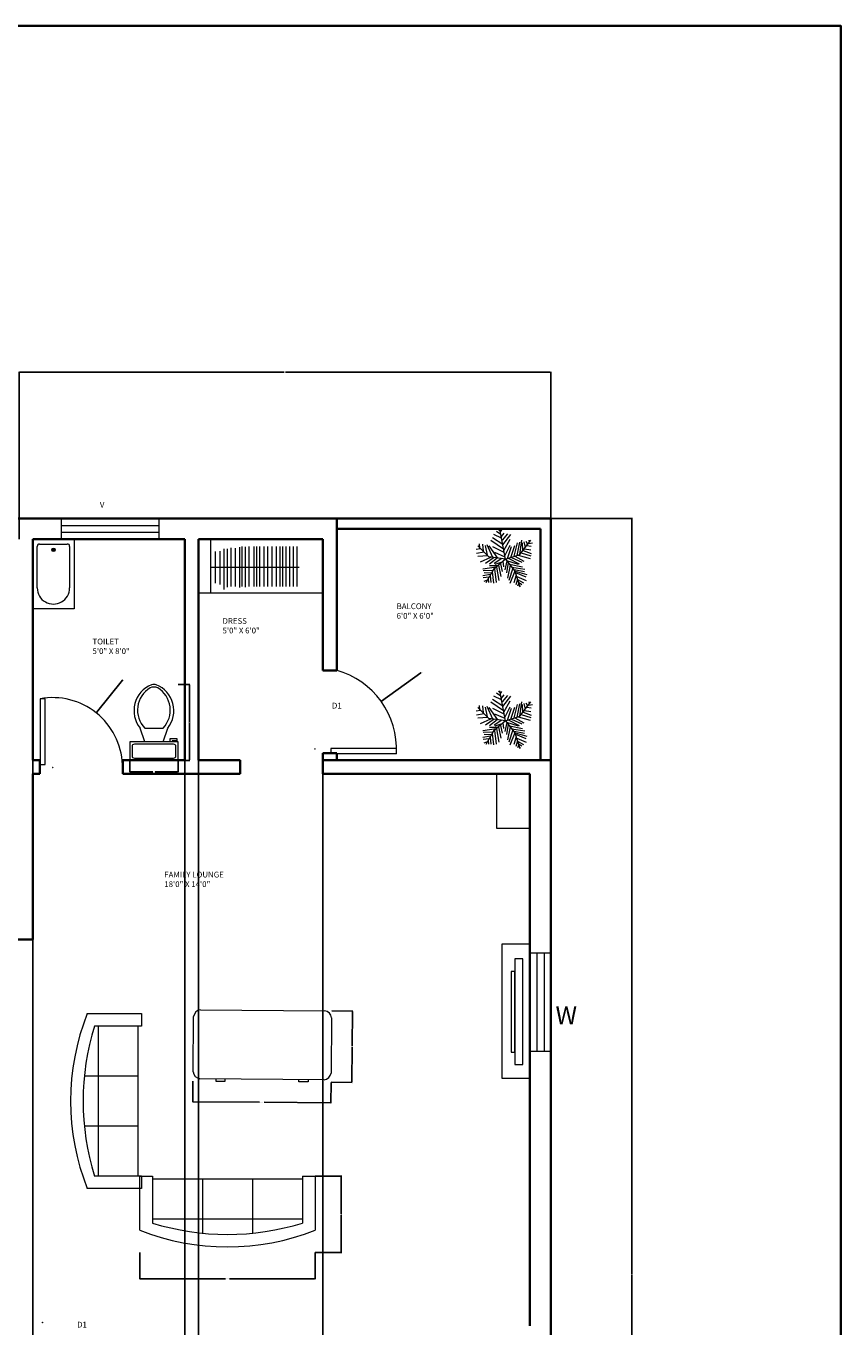
# Model space of a CAD drawing. Units: inches. Extents: x 65 to 1274, y 42 to 1041.
# Tile 6 of 6: x 920 to 1274, y 476 to 1041. Entities that reach past the tile are written whole.
import ezdxf

# ---------------------------------------------------------------- set-up
doc = ezdxf.new("R2010")
doc.units = ezdxf.units.IN
for name, color, linetype, lineweight in [('A-ANNO-DIMS', 2, 'Continuous', 18), ('A-AREA-IDEN', 7, 'Continuous', 18), ('A-DOOR', 3, 'Continuous', 18), ('A-FLOR-CASE', 8, 'Continuous', 18), ('A-FLOR-FIXT', 9, 'Continuous', 18), ('A-FURN', 8, 'Continuous', 18), ('A-GLAZ', 4, 'Continuous', 18), ('A-WALL', 7, 'Continuous', 35), ('L-PLNT', 94, 'Continuous', 13), ('Text', 7, 'Continuous', 18), ('Title Block', 7, 'Continuous', 35)]:
    doc.layers.add(name, color=color, linetype=linetype, lineweight=lineweight)
doc.styles.get("Standard").update_dxf_attribs({"font": 'arial.ttf'})
doc.dimstyles.get("Standard").update_dxf_attribs({"dimtxt": 0.18, "dimasz": 0.18, "dimexe": 0.18, "dimexo": 0.0625, "dimgap": 0.09, "dimtad": 0, "dimtih": 1, "dimtoh": 1, "dimdec": 4, "dimzin": 0, "dimdsep": 46, "dimtxsty": 'Standard', "dimcen": 0.09, "dimadec": 0, "dimazin": 0, "dimtfac": 1, "dimtdec": 4, "dimtofl": 0, "dimtmove": 0, "dimatfit": 3, "dimfxl": 1, "dimtolj": 1, "dimtzin": 0, "dimarcsym": 0})

# ---------------------------------------------------------------- blocks, each defined once
blk = doc.blocks.new('Toilet - top')
for p, q in [((9.5, -6), (9.5, -2)), ((-10, -8.5), (-8, -8.5)), ((-10, -9.5), (-10, -8.5)), ((-7, -9.5), (-10, -9.5)), ((-8, -8.5), (-8, -8)), ((-7, -8), (-7, -9.5)), ((-4, -8), (-6, -14)), ((4, -8), (6, -14)), ((4, -14), (-4, -14))]:
    blk.add_line(p, q)
blk.add_lwpolyline([(10.5, -8), (10.5, 0), (-10.5, 0), (-10.5, -8)], close=True)
for points in [[(-9.5, -2), (-9.5, -6)], [(8.5, -1), (-8.5, -1)], [(-8.5, -7), (8.5, -7)]]:
    blk.add_lwpolyline(points)
for centre, radius, start, end in [((-8.62, -1.88), 0.884, 81.8699, 188.1301), ((8.62, -1.88), 0.884, 351.8699, 98.1301), ((-8.62, -6.12), 0.884, 171.8699, 278.1301), ((8.62, -6.12), 0.884, 261.8699, 8.1301), ((3.52, -21.58), 12.17, 141.4691, 247.9714), ((4.2, -21.82), 11.33, 136.3677, 238.9468), ((-3.52, -21.58), 12.17, 292.0284, 38.5307), ((-4.2, -21.82), 11.33, 301.053, 43.6321), ((0, -27.88), 4, 245.7318, 294.2682), ((0, -29), 4, 254.8605, 285.1395)]:
    blk.add_arc(centre, radius, start, end)
blk = doc.blocks.new('Bath Tub - 26 x 60 in.')
for p, q in [((8, -18), (10, -18)), ((9, -17), (9, -19))]:
    blk.add_line(p, q)
blk.add_lwpolyline([(0, -36), (0, 0), (60, 0), (60, -36)], close=True)
for points in [[(4, -30), (4, -6)], [(6, -4), (42, -4)], [(42, -32), (6, -32)]]:
    blk.add_lwpolyline(points)
for radius in [1.5, 1]:
    blk.add_circle((9, -18), radius)
for centre, radius, start, end in [((5.75, -5.75), 1.77, 81.8699, 188.1301), ((42, -18), 14, 270, 90), ((5.75, -30.25), 1.77, 171.8699, 278.1301)]:
    blk.add_arc(centre, radius, start, end)
blk = doc.blocks.new('Sofa - Roundback 7 ft.')
for p, q in [((-36.000027, -34), (-36.000027, -11.4696)), ((-12.00002, -32.4421), (-12.00003, -6.5971)), ((11.99997, -32.4421), (11.99998, -6.5971)), ((35.99998, -34), (35.99998, -11.4696)), ((-35.999844, -13.3819), (35.9998, -13.3819)), ((-36.000027, -32.4421), (35.99998, -32.4421))]:
    blk.add_line(p, q)
for points in [[(-36.000027, -34), (-42.000027, -34), (-42.000027, -8)], [(41.99998, -8), (41.99998, -34), (35.99998, -34)]]:
    blk.add_lwpolyline(points)
for centre, radius, start, end in [((0, -114.25), 114.25, 68.43141, 111.5686), ((-0.00001, -127.1968), 121.1968, 72.72033, 107.2797)]:
    blk.add_arc(centre, radius, start, end)
blk = doc.blocks.new('Desk - 30 x 60 in.')
for p, q in [((-26.999995, 0), (26.999995, 0)), ((-29.999995, -27), (-29.999995, -3)), ((29.999995, -3), (29.999995, -27)), ((26.999995, -30), (-26.999995, -30)), ((-20.000005, -30), (-20.000005, -31)), ((-20.000005, -31), (-16.000005, -31)), ((-16.000005, -31), (-16.000005, -30)), ((15.999995, -31), (15.999995, -30)), ((19.999995, -31), (15.999995, -31)), ((19.999995, -30), (19.999995, -31))]:
    blk.add_line(p, q)
for centre, start, end in [((-26.499995, -3.5), 98.1301, 171.8699), ((26.499995, -3.5), 8.130102, 81.8699), ((-26.499995, -26.5), 188.1301, 261.8699), ((26.499995, -26.5), 278.1301, 351.8699)]:
    blk.add_arc(centre, 3.535534, start, end)
blk = doc.blocks.new('*U4')
for p, q in [((-8.737, 47.138), (-17.069, 52.711)), ((-10.186, 53.64), (-13.084, 55.962)), ((0, 0), (-10.5, 57)), ((-9.099, 51.782), (-6.563, 55.962)), ((-7.65, 43.423), (-2.578, 49.46)), ((-31.5, 4.5), (-52.5, 25.5)), ((-48.585, 21.131), (-49.309, 29.026)), ((-43.513, 28.561), (-42.427, 15.558)), ((-38.442, 26.239), (-34.819, 7.663)), ((-35.544, 28.097), (-24.314, 3.947)), ((-14.533, 2.09), (-30.834, 25.31)), ((-3.665, 19.273), (-27.574, 35.527)), ((-5.114, 28.097), (-24.676, 40.636)), ((-7.288, 39.707), (-21.778, 46.673)), ((-5.839, 35.992), (4.667, 48.067)), ((-5.114, 27.632), (10.463, 46.673)), ((-2.941, 16.486), (8.652, 37.85)), ((-1.129, 6.734), (9.014, 26.704)), ((10.101, 3.483), (17.708, 26.239)), ((16.259, 5.805), (23.142, 31.348)), ((22.055, 7.198), (27.489, 32.277)), ((27, 9), (48, 36)), ((27.127, 9.056), (31.112, 35.992)), ((31.836, 30.883), (32.561, 16.486)), ((35.096, 32.741), (37.27, 22.524)), ((38.719, 34.134), (41.979, 28.561)), ((40.53, 25.775), (48.862, 24.846)), ((43.791, 29.954), (51.036, 30.883)), ((44.153, 36.456), (45.239, 32.741)), ((-47.498, 19.737), (-55.83, 18.344)), ((-40.615, 13.7), (-55.105, 10.913)), ((-33.37, 6.269), (-52.207, 5.34)), ((-28.299, 3.483), (-47.86, -5.805)), ((-21.416, 3.018), (-38.079, -8.128)), ((0, 0), (-31.5, 4.5)), ((-15.982, 2.09), (-30.11, -9.521)), ((-24.314, 23.917), (-2.941, 13.7)), ((0, 0), (-22.5, -19.5)), ((-6.563, 1.161), (-21.416, -8.128)), ((-20.691, 13.7), (-1.129, 4.876)), ((0, 0), (27, 9)), ((0, 0), (18, -22.5)), ((3.942, 1.625), (11.187, 24.381)), ((6.478, 1.625), (26.04, -8.592)), ((11.187, 3.483), (30.749, -5.805)), ((18.07, 5.805), (35.096, -3.483)), ((24.229, 7.663), (46.688, 1.625)), ((29.662, 12.307), (48.137, 6.269)), ((33.285, 16.486), (48.862, 10.913)), ((36.183, 19.737), (48.137, 17.88)), ((-17.431, -15.094), (-42.789, -18.809)), ((-24.314, -21.596), (-42.427, -22.06)), ((-22.5, -19.5), (-37.5, -45)), ((-15.257, -12.772), (-30.11, -12.772)), ((-25.038, -23.918), (-22.865, -45.281)), ((-20.691, -18.345), (-17.793, -44.352)), ((-6.563, -5.805), (-19.967, -9.985)), ((-17.069, -15.094), (-12.721, -40.172)), ((-13.446, -11.378), (-8.737, -32.741)), ((-9.461, -8.592), (-6.201, -23.453)), ((-4.752, -3.483), (-3.665, -14.629)), ((2.493, -3.019), (-1.491, -20.202)), ((1.769, -2.555), (24.229, -9.521)), ((5.029, -6.27), (2.131, -25.775)), ((9.014, -11.378), (3.58, -35.992)), ((14.085, -16.951), (6.478, -40.172)), ((7.565, -9.056), (32.198, -14.629)), ((18.07, -22.524), (8.289, -45.745)), ((12.274, -15.094), (36.907, -18.809)), ((16.259, -19.738), (36.183, -22.989)), ((18, -22.5), (27, -52.5)), ((18.433, -22.524), (40.53, -29.026)), ((-28.299, -29.026), (-42.789, -31.348)), ((-30.834, -34.135), (-42.427, -35.528)), ((-34.457, -39.708), (-40.978, -42.494)), ((-26.849, -26.24), (-40.253, -25.775)), ((-32.646, -36.921), (-31.921, -44.352)), ((-29.023, -30.884), (-27.936, -43.887)), ((20.244, -30.419), (15.897, -44.816)), ((19.157, -25.311), (38.719, -33.206)), ((22.78, -37.85), (19.519, -48.532)), ((21.331, -32.741), (39.081, -40.636)), ((22.78, -38.314), (34.372, -44.816)), ((24.591, -45.745), (23.142, -50.854)), ((24.591, -43.423), (30.749, -47.603)), ((26.764, -49.925), (28.213, -50.854))]:
    blk.add_line(p, q)
blk = doc.blocks.new('WIN-43-DEEP-FRAME')
for p, q in [((9, 42.65), (0, 42.65)), ((0, 42.65), (0, 0)), ((3, 0), (3, 42.65)), ((6, 42.65), (6, 0)), ((9, 0), (9, 42.65)), ((0, 0), (9, 0))]:
    blk.add_line(p, q)
blk = doc.blocks.new('*D36')
at = {"layer": 'A-ANNO-DIMS', "color": 0, "lineweight": -2, "transparency": 16777216}
for p, q in [((969.32, 508.05), (969.32, 496.52)), ((1045.42, 508.05), (1045.42, 496.52)), ((969.5, 496.7), (1006.47, 496.7)), ((1045.24, 496.7), (1008.28, 496.7))]:
    blk.add_line(p, q, dxfattribs=at)
at = {"layer": 'A-ANNO-DIMS', "color": 0, "transparency": 16777216}
for points in [[(969.5, 496.73), (969.5, 496.67), (969.32, 496.7)], [(1045.24, 496.73), (1045.24, 496.67), (1045.42, 496.7)]]:
    blk.add_solid(points, dxfattribs=at)
at = {"layer": 'Defpoints', "color": 0, "transparency": 16777216}
for p in [(969.32, 508.11), (1045.42, 508.11), (969.32, 496.7)]:
    blk.add_point(p, dxfattribs=at)
at = {"layer": 'A-ANNO-DIMS', "color": 0, "transparency": 16777216, "insert": (1007.37, 496.7), "char_height": 0.18, "attachment_point": 5}
blk.add_mtext('\\A1;SOFA 76 TYP.', dxfattribs=at)
blk = doc.blocks.new('*D37')
at = {"layer": 'A-ANNO-DIMS', "color": 0, "lineweight": -2, "transparency": 16777216}
for p, q in [((1045.48, 541.33), (1057.02, 541.33)), ((1056.84, 541.15), (1056.84, 524.91)), ((1056.84, 508.29), (1056.84, 524.54)), ((1045.48, 508.11), (1057.02, 508.11))]:
    blk.add_line(p, q, dxfattribs=at)
at = {"layer": 'A-ANNO-DIMS', "color": 0, "transparency": 16777216}
for points in [[(1056.81, 541.15), (1056.87, 541.15), (1056.84, 541.33)], [(1056.81, 508.29), (1056.87, 508.29), (1056.84, 508.11)]]:
    blk.add_solid(points, dxfattribs=at)
at = {"layer": 'Defpoints', "color": 0, "transparency": 16777216}
for p in [(1045.42, 541.33), (1045.42, 508.11), (1056.84, 508.11)]:
    blk.add_point(p, dxfattribs=at)
at = {"layer": 'A-ANNO-DIMS', "color": 0, "transparency": 16777216, "insert": (1056.84, 524.72), "char_height": 0.18, "attachment_point": 5}
blk.add_mtext('\\A1;33 TYP.', dxfattribs=at)
blk = doc.blocks.new('*D40')
at = {"layer": 'A-ANNO-DIMS', "color": 0, "lineweight": -2, "transparency": 16777216}
for p, q in [((985.96, 755.09), (991.04, 755.09)), ((990.86, 754.91), (990.86, 738.75)), ((990.86, 722.22), (990.86, 738.38)), ((985.96, 722.04), (991.04, 722.04))]:
    blk.add_line(p, q, dxfattribs=at)
at = {"layer": 'A-ANNO-DIMS', "color": 0, "transparency": 16777216}
for points in [[(990.83, 754.91), (990.89, 754.91), (990.86, 755.09)], [(990.83, 722.22), (990.89, 722.22), (990.86, 722.04)]]:
    blk.add_solid(points, dxfattribs=at)
at = {"layer": 'Defpoints', "color": 0, "transparency": 16777216}
for p in [(985.9, 755.09), (985.9, 722.04), (990.86, 722.04)]:
    blk.add_point(p, dxfattribs=at)
at = {"layer": 'A-ANNO-DIMS', "color": 0, "transparency": 16777216, "insert": (990.86, 738.56), "char_height": 0.18, "attachment_point": 5}
blk.add_mtext('\\A1;WC 33 TYP.', dxfattribs=at)
blk = doc.blocks.new('*D41')
at = {"layer": 'A-ANNO-DIMS', "color": 0, "lineweight": -2, "transparency": 16777216}
for p, q in [((964.9, 721.98), (964.9, 716.9)), ((985.9, 721.98), (985.9, 716.9)), ((965.08, 717.08), (974.87, 717.08)), ((985.72, 717.08), (975.93, 717.08))]:
    blk.add_line(p, q, dxfattribs=at)
at = {"layer": 'A-ANNO-DIMS', "color": 0, "transparency": 16777216}
for points in [[(965.08, 717.11), (965.08, 717.05), (964.9, 717.08)], [(985.72, 717.11), (985.72, 717.05), (985.9, 717.08)]]:
    blk.add_solid(points, dxfattribs=at)
at = {"layer": 'Defpoints', "color": 0, "transparency": 16777216}
for p in [(964.9, 722.04), (985.9, 722.04), (964.9, 717.08)]:
    blk.add_point(p, dxfattribs=at)
at = {"layer": 'A-ANNO-DIMS', "color": 0, "transparency": 16777216, "insert": (975.4, 717.08), "char_height": 0.18, "attachment_point": 5}
blk.add_mtext('\\A1;21 TYP.', dxfattribs=at)
blk = doc.blocks.new('*D42')
at = {"layer": 'A-ANNO-DIMS', "color": 0, "lineweight": -2, "transparency": 16777216}
for p, q in [((992.37, 582.61), (992.29, 573.5)), ((1052.37, 582.07), (1052.29, 572.95)), ((992.47, 573.67), (1021.33, 573.41)), ((1052.11, 573.13), (1023.25, 573.39))]:
    blk.add_line(p, q, dxfattribs=at)
at = {"layer": 'A-ANNO-DIMS', "color": 0, "transparency": 16777216}
for points in [[(992.47, 573.7), (992.47, 573.64), (992.29, 573.68)], [(1052.11, 573.16), (1052.11, 573.1), (1052.29, 573.13)]]:
    blk.add_solid(points, dxfattribs=at)
at = {"layer": 'Defpoints', "color": 0, "transparency": 16777216}
for p in [(992.37, 582.67), (1052.37, 582.13), (1052.29, 573.13)]:
    blk.add_point(p, dxfattribs=at)
at = {"layer": 'A-ANNO-DIMS', "color": 0, "transparency": 16777216, "insert": (1022.29, 573.4), "char_height": 0.18, "attachment_point": 5}
blk.add_mtext('\\A1;TABLE 60 TYP.', dxfattribs=at)
blk = doc.blocks.new('*D43')
at = {"layer": 'A-ANNO-DIMS', "color": 0, "lineweight": -2, "transparency": 16777216}
for p, q in [((1052.71, 613.13), (1061.83, 613.04)), ((1061.65, 612.87), (1061.51, 597.73)), ((1061.37, 582.23), (1061.51, 597.36)), ((1052.43, 582.13), (1061.55, 582.05))]:
    blk.add_line(p, q, dxfattribs=at)
at = {"layer": 'A-ANNO-DIMS', "color": 0, "transparency": 16777216}
for points in [[(1061.62, 612.87), (1061.68, 612.87), (1061.65, 613.05)], [(1061.34, 582.23), (1061.4, 582.23), (1061.37, 582.05)]]:
    blk.add_solid(points, dxfattribs=at)
at = {"layer": 'Defpoints', "color": 0, "transparency": 16777216}
for p in [(1052.65, 613.13), (1061.65, 613.05), (1052.37, 582.13)]:
    blk.add_point(p, dxfattribs=at)
at = {"layer": 'A-ANNO-DIMS', "color": 0, "transparency": 16777216, "insert": (1061.51, 597.55), "char_height": 0.18, "attachment_point": 5}
blk.add_mtext('\\A1;31 TYP.', dxfattribs=at)
blk = doc.blocks.new('*D65')
at = {"layer": 'A-ANNO-DIMS', "color": 0, "lineweight": -2, "transparency": 16777216}
for p, q in [((1147.89, 827.15), (1183.32, 827.15)), ((1183.14, 826.97), (1183.14, 498.83)), ((1183.14, 170.33), (1183.14, 498.47)), ((1147.89, 170.15), (1183.32, 170.15))]:
    blk.add_line(p, q, dxfattribs=at)
at = {"layer": 'A-ANNO-DIMS', "color": 0, "transparency": 16777216}
for points in [[(1183.11, 826.97), (1183.17, 826.97), (1183.14, 827.15)], [(1183.11, 170.33), (1183.17, 170.33), (1183.14, 170.15)]]:
    blk.add_solid(points, dxfattribs=at)
at = {"layer": 'Defpoints', "color": 0, "transparency": 16777216}
for p in [(1147.83, 827.15), (1183.14, 827.15), (1147.83, 170.15)]:
    blk.add_point(p, dxfattribs=at)
at = {"layer": 'A-ANNO-DIMS', "color": 0, "transparency": 16777216, "insert": (1183.14, 498.65), "char_height": 0.18, "attachment_point": 5}
blk.add_mtext('\\A1;657', dxfattribs=at)
blk = doc.blocks.new('*D67')
at = {"layer": 'A-ANNO-DIMS', "color": 0, "lineweight": -2, "transparency": 16777216}
for p, q in [((916.83, 818.21), (916.83, 890.96)), ((917.01, 890.78), (1032.06, 890.78)), ((1147.65, 890.78), (1032.6, 890.78)), ((1147.83, 827.21), (1147.83, 890.96))]:
    blk.add_line(p, q, dxfattribs=at)
at = {"layer": 'A-ANNO-DIMS', "color": 0, "transparency": 16777216}
for points in [[(917.01, 890.81), (917.01, 890.75), (916.83, 890.78)], [(1147.65, 890.81), (1147.65, 890.75), (1147.83, 890.78)]]:
    blk.add_solid(points, dxfattribs=at)
at = {"layer": 'Defpoints', "color": 0, "transparency": 16777216}
for p in [(1147.83, 890.78), (1147.83, 827.15), (916.83, 818.15)]:
    blk.add_point(p, dxfattribs=at)
at = {"layer": 'A-ANNO-DIMS', "color": 0, "transparency": 16777216, "insert": (1032.33, 890.78), "char_height": 0.18, "attachment_point": 5}
blk.add_mtext('\\A1;231', dxfattribs=at)
blk = doc.blocks.new('*D68')
at = {"layer": 'A-ANNO-DIMS', "color": 0, "lineweight": -2, "transparency": 16777216}
for p, q in [((922.83, 722.09), (922.83, 134.18)), ((988.83, 722.09), (988.83, 134.18)), ((923.01, 134.36), (955.61, 134.36)), ((988.65, 134.36), (956.05, 134.36))]:
    blk.add_line(p, q, dxfattribs=at)
at = {"layer": 'A-ANNO-DIMS', "color": 0, "transparency": 16777216}
for points in [[(923.01, 134.39), (923.01, 134.33), (922.83, 134.36)], [(988.65, 134.39), (988.65, 134.33), (988.83, 134.36)]]:
    blk.add_solid(points, dxfattribs=at)
at = {"layer": 'Defpoints', "color": 0, "transparency": 16777216}
for p in [(922.83, 722.15), (988.83, 722.15), (988.83, 134.36)]:
    blk.add_point(p, dxfattribs=at)
at = {"layer": 'A-ANNO-DIMS', "color": 0, "transparency": 16777216, "insert": (955.83, 134.36), "char_height": 0.18, "attachment_point": 5}
blk.add_mtext('\\A1;66', dxfattribs=at)
blk = doc.blocks.new('*D69')
at = {"layer": 'A-ANNO-DIMS', "color": 0, "lineweight": -2, "transparency": 16777216}
for p, q in [((994.83, 722.09), (994.83, 134.18)), ((1048.83, 722.09), (1048.83, 134.18)), ((995.01, 134.36), (1021.61, 134.36)), ((1048.65, 134.36), (1022.05, 134.36))]:
    blk.add_line(p, q, dxfattribs=at)
at = {"layer": 'A-ANNO-DIMS', "color": 0, "transparency": 16777216}
for points in [[(995.01, 134.39), (995.01, 134.33), (994.83, 134.36)], [(1048.65, 134.39), (1048.65, 134.33), (1048.83, 134.36)]]:
    blk.add_solid(points, dxfattribs=at)
at = {"layer": 'Defpoints', "color": 0, "transparency": 16777216}
for p in [(994.83, 722.15), (1048.83, 722.15), (1048.83, 134.36)]:
    blk.add_point(p, dxfattribs=at)
at = {"layer": 'A-ANNO-DIMS', "color": 0, "transparency": 16777216, "insert": (1021.83, 134.36), "char_height": 0.18, "attachment_point": 5}
blk.add_mtext('\\A1;54', dxfattribs=at)
blk = doc.blocks.new('*D82')
at = {"layer": 'A-ANNO-DIMS', "color": 0, "lineweight": -2, "transparency": 16777216}
for p, q in [((961.69, 756.91), (950.45, 742.83)), ((961.87, 756.91), (961.69, 756.91)), ((931.33, 718.98), (931.51, 718.98)), ((931.42, 718.89), (931.42, 719.07))]:
    blk.add_line(p, q, dxfattribs=at)
at = {"layer": 'A-ANNO-DIMS', "color": 0, "transparency": 16777216}
blk.add_solid([(950.43, 742.85), (950.48, 742.81), (950.34, 742.69)], dxfattribs=at)
at = {"layer": 'Defpoints', "color": 0, "transparency": 16777216}
for p in [(950.34, 742.69), (931.42, 718.98)]:
    blk.add_point(p, dxfattribs=at)
at = {"layer": 'A-ANNO-DIMS', "color": 0, "transparency": 16777216, "insert": (962.42, 756.91), "char_height": 0.18, "attachment_point": 5}
blk.add_mtext('\\A1;R30.327', dxfattribs=at)
blk = doc.blocks.new('*D83')
at = {"layer": 'A-ANNO-DIMS', "color": 0, "lineweight": -2, "transparency": 16777216}
for p, q in [((1091.41, 760.12), (1074.3, 747.81)), ((1091.59, 760.12), (1091.41, 760.12)), ((1045.31, 727.01), (1045.49, 727.01)), ((1045.4, 726.92), (1045.4, 727.1))]:
    blk.add_line(p, q, dxfattribs=at)
at = {"layer": 'A-ANNO-DIMS', "color": 0, "transparency": 16777216}
blk.add_solid([(1074.28, 747.83), (1074.32, 747.79), (1074.16, 747.7)], dxfattribs=at)
at = {"layer": 'Defpoints', "color": 0, "transparency": 16777216}
for p in [(1074.16, 747.7), (1045.4, 727.01)]:
    blk.add_point(p, dxfattribs=at)
at = {"layer": 'A-ANNO-DIMS', "color": 0, "transparency": 16777216, "insert": (1092.06, 760.12), "char_height": 0.18, "attachment_point": 5}
blk.add_mtext('\\A1;R35.42', dxfattribs=at)
blk = doc.blocks.new('*D85')
at = {"layer": 'A-ANNO-DIMS', "color": 0, "lineweight": -2, "transparency": 16777216}
for p, q in [((926.86, 477.66), (927.04, 477.66)), ((926.95, 477.57), (926.95, 477.75)), ((964.73, 436.07), (950.68, 451.53)), ((964.91, 436.07), (964.73, 436.07))]:
    blk.add_line(p, q, dxfattribs=at)
at = {"layer": 'A-ANNO-DIMS', "color": 0, "transparency": 16777216}
blk.add_solid([(950.7, 451.55), (950.66, 451.51), (950.56, 451.66)], dxfattribs=at)
at = {"layer": 'Defpoints', "color": 0, "transparency": 16777216}
for p in [(926.95, 477.66), (950.56, 451.66)]:
    blk.add_point(p, dxfattribs=at)
at = {"layer": 'A-ANNO-DIMS', "color": 0, "transparency": 16777216, "insert": (965.46, 436.07), "char_height": 0.18, "attachment_point": 5}
blk.add_mtext('\\A1;R35.115', dxfattribs=at)

msp = doc.modelspace()

# ---------------------------------------------------------------- linework, layer by layer
at = {"layer": 'A-DOOR'}
for points in [[(925.9485, 720.2146), (928.2059, 720.2146), (928.2059, 748.7361), (925.9485, 748.7361)], [(1080.7606, 724.9938), (1080.7606, 727.2511), (1052.239, 727.2511), (1052.239, 724.9938)]]:
    msp.add_lwpolyline(points, close=True, dxfattribs=at)
for centre, radius, start, end in [((1045.4048, 727.013), 35.422, 356.63948, 74.843363), ((931.4225, 718.9837), 30.3267, 2.40638, 100.40835)]:
    msp.add_arc(centre, radius, start, end, dxfattribs=at)
at = {"layer": 'A-FLOR-CASE'}
for p, q in [((999.9793, 818.1476), (999.9793, 794.8948)), ((1005.7493, 813.9539), (1005.7493, 796.3693)), ((1007.2346, 814.011), (1007.2346, 797.3399)), ((1008.8342, 814.4677), (1008.8342, 797.6253)), ((1010.7195, 814.2393), (1010.7195, 797.6253)), ((1012.6619, 814.7532), (1012.6619, 797.1686)), ((1013.633, 814.9815), (1013.633, 797.6253)), ((1015.0041, 814.8674), (1015.0041, 797.2828)), ((1016.718, 814.9815), (1016.718, 797.6253)), ((1018.7746, 814.9815), (1018.7746, 797.6253)), ((1019.9743, 814.9815), (1019.9743, 797.6253)), ((1021.2883, 814.9815), (1021.2883, 797.6253)), ((1023.2306, 814.9815), (1023.2306, 797.6253)), ((1024.8302, 814.9815), (1024.8302, 797.6253)), ((1026.6583, 814.9815), (1026.6583, 797.6253)), ((1028.4865, 814.9815), (1028.4865, 797.6253)), ((1030.1432, 814.9815), (1030.1432, 797.6253)), ((1031.2858, 814.9815), (1031.2858, 797.6253)), ((1032.7711, 814.9815), (1032.7711, 797.6253)), ((1034.3136, 814.9815), (1034.3136, 797.6253)), ((1035.8561, 814.9815), (1035.8561, 797.6253)), ((1037.5699, 814.9815), (1037.5699, 797.6253)), ((1002.0931, 812.8691), (1002.0931, 799.1097)), ((1004.0926, 812.9833), (1004.0926, 798.4246)), ((1000.0364, 806.0751), (1038.5982, 806.0751)), ((994.8297, 794.8948), (1048.7467, 794.8948))]:
    msp.add_line(p, q, dxfattribs=at)
at = {"layer": 'A-FURN'}
for points in [[(1139.1108, 715.9482), (1124.3115, 715.9482), (1124.3115, 692.5956), (1139.1108, 692.5956)], [(1138.7293, 642.1051), (1126.6276, 642.1051), (1126.6276, 583.8702), (1138.7293, 583.8702)], [(1135.6784, 635.7023), (1132.2208, 635.7023), (1132.2208, 589.7648), (1135.6784, 589.7648)], [(1132.1777, 630.2711), (1130.6508, 630.2711), (1130.6508, 595.1758), (1132.1777, 595.1758)]]:
    msp.add_lwpolyline(points, close=True, dxfattribs=at)
at = {"layer": 'A-WALL'}
for p, q in [((763.8298, 827.1476), (1147.8298, 827.1476)), ((1054.8298, 761.1476), (1054.8298, 827.1476)), ((1147.8298, 827.1476), (1147.8298, 170.1476)), ((1054.8298, 822.6476), (1143.3298, 822.6476)), ((1143.3298, 822.6476), (1143.3298, 722.1476)), ((922.8297, 818.1476), (922.8297, 722.1476)), ((922.8297, 722.1476), (922.8297, 818.1476)), ((922.8297, 818.1476), (988.8297, 818.1476)), ((988.8297, 722.1476), (988.8297, 818.1476)), ((988.8297, 818.1476), (988.8297, 722.1476)), ((994.8297, 818.1476), (994.8297, 722.1476)), ((994.8297, 818.1476), (1048.8298, 818.1476)), ((1048.8298, 761.1476), (1048.8298, 818.1476)), ((1048.8298, 761.1476), (1054.8298, 761.1476)), ((1048.8298, 716.1476), (1048.8298, 725.1476)), ((1048.8298, 725.1476), (1054.8298, 725.1476)), ((1054.8298, 722.1476), (1054.8298, 725.1476)), ((922.8297, 722.1476), (925.8298, 722.1476)), ((925.8298, 722.1476), (925.8298, 716.1476)), ((961.8298, 722.1476), (988.8297, 722.1476)), ((961.8298, 722.1476), (961.8298, 716.1476)), ((994.8297, 722.1476), (1012.8298, 722.1476)), ((1012.8298, 716.1476), (1012.8298, 722.1476)), ((1048.8298, 722.1476), (1147.8298, 722.1476)), ((922.8297, 716.1476), (925.8298, 716.1476)), ((922.8297, 716.1476), (922.8297, 644.1476)), ((922.8297, 644.1476), (922.8297, 716.1476)), ((961.8298, 716.1476), (1012.8298, 716.1476)), ((1048.8298, 716.1476), (1138.8298, 716.1476)), ((1138.8298, 716.1476), (1138.8298, 476.1476)), ((913.8298, 644.1476), (922.8297, 644.1476))]:
    msp.add_line(p, q, dxfattribs=at)
at = {"layer": 'Title Block'}
msp.add_lwpolyline([(64.7421, 1041.286), (1273.976, 1041.286), (1273.976, 41.6396), (64.7421, 41.6396)], close=True, dxfattribs=at)

# ---------------------------------------------------------------- block references
at = {"layer": 'A-FLOR-FIXT', "xscale": 0.5021616587859374, "yscale": 0.5021616587859374, "zscale": 0.5021616587859374, "rotation": 270}
msp.add_blockref('Bath Tub - 26 x 60 in.', (940.7903, 818.0843), dxfattribs=at)
at = {"layer": 'A-FLOR-FIXT', "rotation": 180}
msp.add_blockref('Toilet - top', (975.4023, 722.0389), dxfattribs=at)
at = {"layer": 'A-FURN', "xscale": 0.9059646076568906, "yscale": 0.9059646076568906, "zscale": 0.9059646076568906}
for p, rotation in [((939.2077, 573.927), 89.99999999999996), ((1007.3715, 510.5308), 180)]:
    msp.add_blockref('Sofa - Roundback 7 ft.', p, dxfattribs=dict(at, rotation=rotation))
at = {"layer": 'A-FURN', "rotation": 359.4788228304995}
msp.add_blockref('Desk - 30 x 60 in.', (1022.6525, 613.4007), dxfattribs=at)
at = {"layer": 'A-GLAZ'}
for p, rotation in [((935.0488, 827.136), 270), ((1147.9357, 638.2779), 180)]:
    msp.add_blockref('WIN-43-DEEP-FRAME', p, dxfattribs=dict(at, rotation=rotation))
at = {"layer": 'L-PLNT', "xscale": 0.2291951906982327, "yscale": 0.2291951906982327, "zscale": 0.2291951906982327}
for p in [(1128.1705, 809.4742), (1128.1705, 739.1969)]:
    msp.add_blockref('*U4', p, dxfattribs=at)

# ---------------------------------------------------------------- texts
at = {"layer": 'A-AREA-IDEN', "char_height": 2.5, "attachment_point": 1}
for s, width, insert in [('BALCONY\\P6\'0" X 6\'0"', 32.971432, (1080.8835, 790.2842)), ('DRESS\\P5\'0" X 6\'0"', 25.048063, (1005.2281, 783.8984)), ('TOILET\\P5\'0" X 8\'0"', 16.613509, (948.7225, 774.9474)), ('FAMILY LOUNGE\\P18\'0" X 14\'0"', 71.565891, (979.9265, 673.6281))]:
    msp.add_mtext_dynamic_manual_height_columns(s, width=width, gutter_width=12.5, heights=[0], dxfattribs=dict(at, insert=insert))
at = {"layer": 'Text', "attachment_point": 1}
for s, width, gutter_width, insert, char_height in [('V', 5.099062, 12.5, (951.925, 834.3666), 2.5), ('D1', 17.380293, 12.5, (1052.7812, 747.0777), 2.5), ('W', 96.254197, 39.1027, (1149.9147, 615.1489), 7.8205), ('D1', 7.191641, 12.5, (942.0183, 477.9874), 2.5)]:
    msp.add_mtext_dynamic_manual_height_columns(s, width=width, gutter_width=gutter_width, heights=[0], dxfattribs=dict(at, insert=insert, char_height=char_height))

# ---------------------------------------------------------------- dimensions: what is measured, and where the dimension line sits
at = {"layer": 'A-ANNO-DIMS'}
for base, p1, p2, picture, middle in [((1147.8298, 890.7807), (916.8297, 818.1476), (1147.8298, 827.1476), '*D67', (1032.3298, 890.7807)), ((988.8297, 134.3565), (922.8297, 722.1476), (988.8297, 722.1476), '*D68', (955.8297, 134.3565)), ((1048.8298, 134.3565), (994.8297, 722.1476), (1048.8298, 722.1476), '*D69', (1021.8297, 134.3565))]:
    dim = msp.add_linear_dim(base=base, p1=p1, p2=p2, dimstyle='Standard', override={"dimdec": 0, "dimlfac": 1, "dimrnd": 0, "dimzin": 0, "dimdsep": 46, "dimlunit": 2}, dxfattribs=at)
    dim.commit()
    dim.dimension.update_dxf_attribs({"geometry": picture, "text_midpoint": middle})
dim = msp.add_linear_dim(base=(1183.1357, 827.1476), p1=(1147.8298, 170.1476), p2=(1147.8298, 827.1476), angle=90, dimstyle='Standard', override={"dimdec": 0, "dimlfac": 1, "dimrnd": 0, "dimzin": 0, "dimdsep": 46, "dimlunit": 2}, dxfattribs=at)
dim.commit()
dim.dimension.update_dxf_attribs({"geometry": '*D65', "text_midpoint": (1183.1357, 498.6476)})
for center, mpoint, override, picture, middle in [((1045.4048, 727.013), (1074.1554, 747.7043), {"dimdec": 2, "dimlfac": 1, "dimrnd": 0, "dimzin": 0, "dimdsep": 46, "dimlunit": 2}, '*D83', (1092.0646, 760.119)), ((931.4225, 718.9837), (950.3399, 742.6869), {"dimdec": 3, "dimlfac": 1, "dimrnd": 0, "dimzin": 0, "dimdsep": 46, "dimlunit": 2}, '*D82', (962.4201, 756.9088)), ((926.948, 477.6553), (950.5612, 451.6648), {"dimdec": 3, "dimlfac": 1, "dimrnd": 0, "dimzin": 0, "dimdsep": 46, "dimlunit": 2}, '*D85', (965.4596, 436.0704))]:
    dim = msp.add_radius_dim(center=center, mpoint=mpoint, dimstyle='Standard', override=override, dxfattribs=at)
    dim.commit()
    dim.dimension.update_dxf_attribs({"geometry": picture, "text_midpoint": middle, "dimtype": 164})
for base, p1, p2, angle, text, picture, middle in [((990.8592, 722.0389), (985.9023, 755.0852), (985.9023, 722.0389), 270, 'WC <> TYP.', '*D40', (990.8592, 738.5621)), ((964.9023, 717.082), (985.9023, 722.0389), (964.9023, 722.0389), 180, '<> TYP.', '*D41', (975.4023, 717.082)), ((1061.6509, 613.0459), (1052.3693, 582.1291), (1052.6513, 613.1278), 89.478823, '<> TYP.', '*D43', (1061.5099, 597.5466)), ((1052.2874, 573.1295), (992.3718, 582.6749), (1052.3693, 582.1291), 359.478823, 'TABLE <> TYP.', '*D42', (1022.2887, 573.4023)), ((1056.8372, 508.1148), (1045.422, 541.3335), (1045.422, 508.1148), 270, '<> TYP.', '*D37', (1056.8372, 524.7242)), ((969.321, 496.6997), (1045.422, 508.1148), (969.321, 508.1148), 180, 'SOFA <> TYP.', '*D36', (1007.3715, 496.6997))]:
    dim = msp.add_linear_dim(base=base, p1=p1, p2=p2, angle=angle, text=text, dimstyle='Standard', override={"dimdec": 0, "dimlfac": 1, "dimrnd": 0, "dimzin": 0, "dimdsep": 46, "dimlunit": 2}, dxfattribs=at)
    dim.commit()
    dim.dimension.update_dxf_attribs({"geometry": picture, "text_midpoint": middle})

doc.saveas('drawing.dxf')
